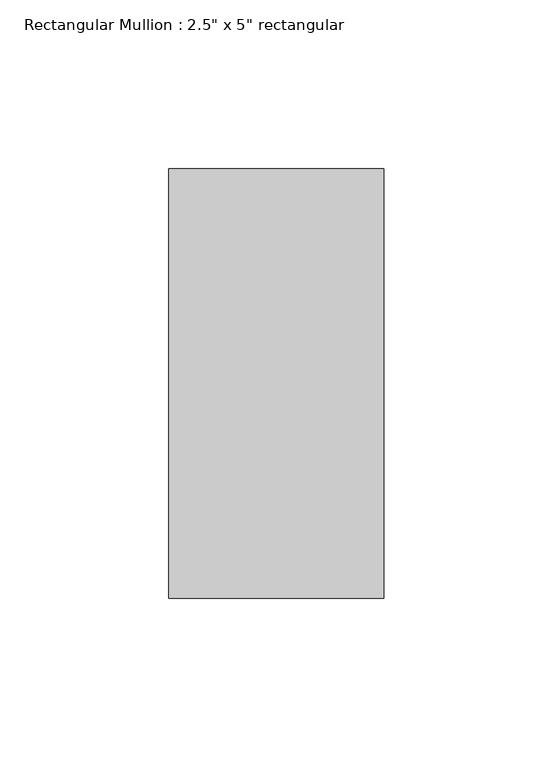
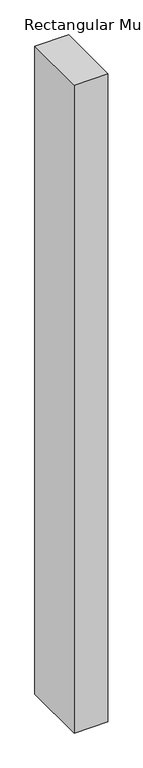
"""IFC4 building model written with IfcOpenShell, lengths in millimetres: member geometry."""

from ifc_helpers import new_model, si_unit, frame, origin, place, context, project, spatial, polyline, outline, extrude, source, transform, mapped, element, save


def member_f10a135f(model_context):
    return source(origin(), model_context, "Body", "SweptSolid", [
        extrude(outline(polyline([(31.75, 63.5), (31.75, -63.5), (-31.75, -63.5), (-31.75, 63.5), (31.75, 63.5)])), frame((0.0, 0.0, -1282.9185959), z_axis=(0.0, 0.0, 1.0), x_axis=(1.0, 0.0, 0.0)), (0.0, 0.0, 1.0), 1282.9185959),
    ])


if __name__ == "__main__":
    model = new_model("IFC4")
    model_context = context("Model", 3, world=origin())
    ifc_project = project(units=[si_unit("LENGTHUNIT", "METRE", prefix="MILLI")], contexts=[model_context])
    site = spatial("IfcSite", under=ifc_project)
    building = spatial("IfcBuilding", under=site)
    placement = place(None, origin())
    member_shape = member_f10a135f(model_context)
    element("IfcMember", 1, ObjectType="Rectangular Mullion : 2.5\" x 5\" rectangular", at=placement, inside=building, context=model_context, shape_type="MappedRepresentation", body=[
        mapped(member_shape, transform((0.0, 0.0, 0.0), x_axis=(1.0, 0.0, 0.0), y_axis=(0.0, 1.0, 0.0), z_axis=(0.0, 0.0, 1.0))),
    ])
    save(model, "model.ifc")

# Revit data of these elements
# Type "Rectangular Mullion : 2.5\" x 5\" rectangular"
#   built-in parameter 1007304 = 0.416667 (stored number, unit not read)
#   built-in parameter 1007301 = 0.104167 (stored number, unit not read)
#   built-in parameter 1007300 = 0.104167 (stored number, unit not read)
# Element 1 (IfcMember, "Rectangular Mullion : 2.5\" x 5\" rectangular")
#   Materials on its faces: "Aluminum"
# Materials
#   "Aluminum": class "Metal", colour RGB 247 247 247, transparency 0, Description = "Aluminum 6061", Cost = 0
